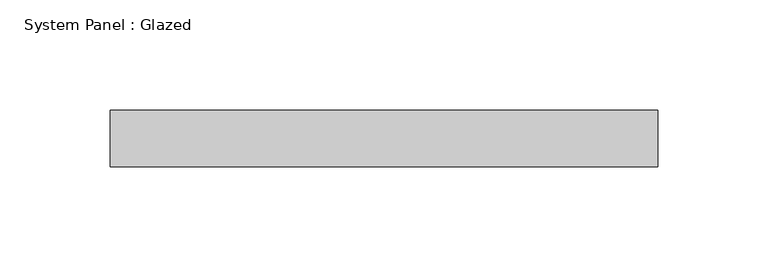
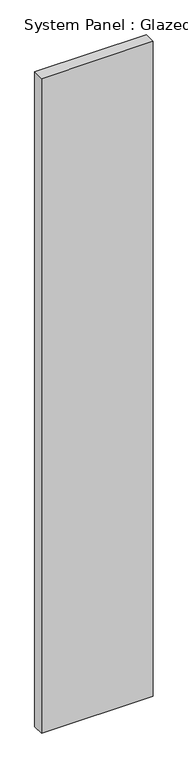
"""IFC4 building model written with IfcOpenShell, lengths in millimetres: plate geometry, System Panel : Glazed."""

from ifc_helpers import new_model, si_unit, origin, origin_with_axes, place, context, project, spatial, polyline, outline, extrude, source, transform, mapped, element, save


def system_panel_glazed_5a7f8ff5(model_context):
    return source(origin(), model_context, "Body", "SweptSolid", [
        extrude(outline(polyline([(123.825, 19.05), (-123.825, 19.05), (-123.825, 44.45), (123.825, 44.45), (123.825, 19.05)])), origin_with_axes(), (0.0, 0.0, 1.0), 1532.4287133),
    ])


if __name__ == "__main__":
    model = new_model("IFC4")
    model_context = context("Model", 3, world=origin())
    ifc_project = project(units=[si_unit("LENGTHUNIT", "METRE", prefix="MILLI")], contexts=[model_context])
    site = spatial("IfcSite", under=ifc_project)
    building = spatial("IfcBuilding", under=site)
    placement = place(None, origin())
    system_panel_glazed_shape = system_panel_glazed_5a7f8ff5(model_context)
    element("IfcPlate", 1, ObjectType="System Panel : Glazed", at=placement, inside=building, context=model_context, shape_type="MappedRepresentation", body=[
        mapped(system_panel_glazed_shape, transform((0.0, 0.0, 0.0), x_axis=(1.0, 0.0, 0.0), y_axis=(0.0, 1.0, 0.0), z_axis=(0.0, 0.0, 1.0))),
    ])
    save(model, "model.ifc")

# Revit data of these elements
# Type "System Panel : Glazed"
#   Construction Type Id = "GSP4R"
#   Analytic Construction = "1/8 in Pilkington single glazing"
#   Visual Light Transmittance = 0.9
#   Solar Heat Gain Coefficient = 0.86
#   Heat Transfer Coefficient (U) = 1.18115 BTU/(h·ft²·°F)
#   Define Thermal Properties by = 1
# Element 1 (IfcPlate, "System Panel : Glazed")
#   Materials on its faces: "Glass"
# Materials
#   "Glass": class "Glass", colour RGB 0 128 192, transparency 0.75, Description = "Soda Lime Glass", Cost = 0
